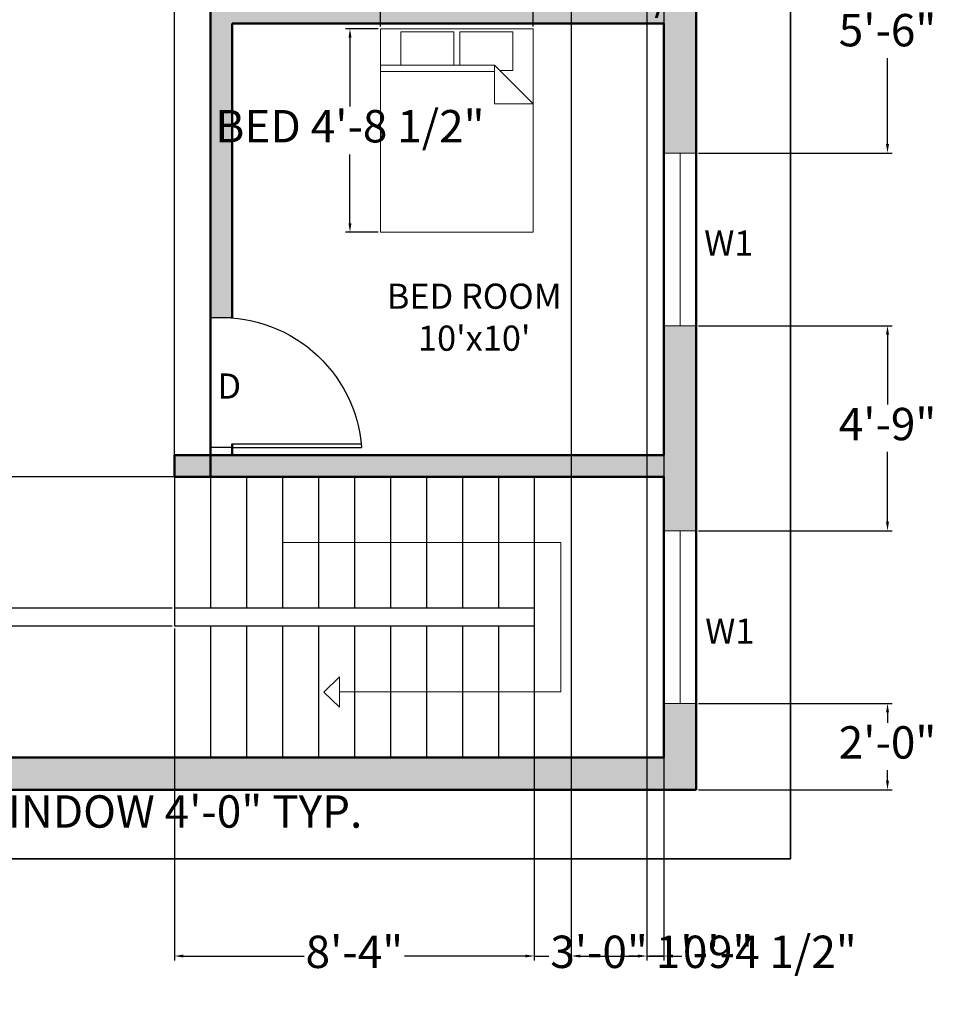
# Model space of a CAD drawing. Units: inches. Extents: x 6193 to 6719, y 6945 to 7563.
# Tile 2 of 4: x 6464 to 6719, y 6945 to 7219. Entities that reach past the tile are written whole.
import ezdxf

# ---------------------------------------------------------------- set-up
doc = ezdxf.new("R2010")
doc.units = ezdxf.units.IN
for name, color, linetype, lineweight in [('A-ANNO-DIMS', 2, 'Continuous', 18), ('A-ANNO-SYMB', 7, 'Continuous', 18), ('A-ANNO-TEXT', 7, 'Continuous', 18), ('A-ANNO-TTLB', 7, 'Continuous', 35), ('A-AREA-IDEN', 7, 'Continuous', 25), ('A-DOOR', 3, 'Continuous', 25), ('A-FLOR-STRS', 7, 'Continuous', 25), ('A-FURN', 8, 'Continuous', 18), ('A-GLAZ', 4, 'Continuous', 18), ('A-WALL', 7, 'Continuous', 50)]:
    doc.layers.add(name, color=color, linetype=linetype, lineweight=lineweight)
doc.layers.add('A-WALL-PATT', color=18, linetype='Continuous', lineweight=13, true_color=0x000000)
doc.styles.get("Standard").update_dxf_attribs({"font": 'arial.ttf'})
doc.dimstyles.new('ISO-25', dxfattribs={"dimtxt": 9, "dimasz": 2.5, "dimexe": 1.25, "dimexo": 0.625, "dimgap": 2, "dimtad": 0, "dimtih": 1, "dimtoh": 1, "dimdec": 1, "dimlunit": 4, "dimtxsty": 'Standard', "dimcen": 2.5, "dimadec": 0, "dimazin": 0, "dimtfac": 0.5, "dimtdec": 1, "dimtmove": 0, "dimatfit": 3, "dimfxl": 1, "dimarcsym": 0})

# ---------------------------------------------------------------- blocks, each defined once
blk = doc.blocks.new('Bed - Queen')
for p, q in [((0, -80.00003), (0, 0)), ((0, 0), (59.99999, 0)), ((59.99999, 0), (59.99999, -80.00003)), ((7.99999, -1.2), (28.79998, -1.2)), ((7.99999, -14.4), (7.99999, -1.2)), ((28.79998, -1.2), (28.79998, -14.4)), ((31.19999, -1.2), (51.99999, -1.2)), ((31.19999, -14.4), (31.19999, -1.2)), ((51.99999, -1.2), (51.99999, -16.4)), ((0, -14.4), (44.8, -14.4)), ((59.99999, -29.6), (44.8, -14.4)), ((44.8, -14.4), (44.8, -29.6)), ((44.8, -16.8), (0, -16.8)), ((51.99999, -16.4), (46.79936, -16.4)), ((44.8, -29.6), (59.99999, -29.6)), ((59.99999, -80.00003), (0, -80.00003))]:
    blk.add_line(p, q)
blk = doc.blocks.new('DOOR-SWING-36IN')
for p, q in [((0, 6), (0, 42)), ((1, 6), (1, 41.91)), ((0, 6), (0, 0)), ((36, 6), (36, 0))]:
    blk.add_line(p, q)
blk.add_arc((-3, 3), 39.12, 355.6013, 85.6013)
blk = doc.blocks.new('WIN-48IN')
for p, q in [((0, 48), (9, 48)), ((4.5, 48), (4.5, 0)), ((0, 0), (9, 0))]:
    blk.add_line(p, q)
blk = doc.blocks.new('*D14')
at = {"layer": 'A-ANNO-DIMS', "color": 0, "lineweight": -2, "transparency": 16777216}
for p, q in [((6395.41, 7004.04), (6395.41, 6996.21)), ((6443.41, 7004.04), (6443.41, 6996.21)), ((6397.91, 6997.46), (6440.91, 6997.46)), ((6443.41, 6997.46), (6445.91, 6997.46))]:
    blk.add_line(p, q, dxfattribs=at)
at = {"layer": 'A-ANNO-DIMS', "color": 0, "transparency": 16777216}
for points in [[(6397.91, 6997.88), (6397.91, 6997.05), (6395.41, 6997.46)], [(6440.91, 6997.88), (6440.91, 6997.05), (6443.41, 6997.46)]]:
    blk.add_solid(points, dxfattribs=at)
at = {"layer": 'Defpoints', "color": 0, "transparency": 16777216}
for p in [(6395.41, 7004.66), (6443.41, 7004.66), (6443.41, 6997.46)]:
    blk.add_point(p, dxfattribs=at)
at = {"layer": 'A-ANNO-DIMS', "color": 0, "transparency": 16777216, "insert": (6504.85, 6997.46), "char_height": 9, "attachment_point": 5}
blk.add_mtext('WINDOW 4\'-0" TYP.', dxfattribs=at)
blk = doc.blocks.new('*D18')
at = {"layer": 'A-ANNO-DIMS', "color": 0, "lineweight": -2, "transparency": 16777216}
for p, q in [((6563.91, 7216.24), (6554.8, 7216.24)), ((6556.05, 7213.74), (6556.05, 7194.61)), ((6556.05, 7162.17), (6556.05, 7181.3)), ((6563.91, 7159.67), (6554.8, 7159.67))]:
    blk.add_line(p, q, dxfattribs=at)
at = {"layer": 'A-ANNO-DIMS', "color": 0, "transparency": 16777216}
for points in [[(6555.64, 7213.74), (6556.47, 7213.74), (6556.05, 7216.24)], [(6555.64, 7162.17), (6556.47, 7162.17), (6556.05, 7159.67)]]:
    blk.add_solid(points, dxfattribs=at)
at = {"layer": 'Defpoints', "color": 0, "transparency": 16777216}
for p in [(6556.05, 7216.24), (6564.54, 7216.24), (6564.54, 7159.67)]:
    blk.add_point(p, dxfattribs=at)
at = {"layer": 'A-ANNO-DIMS', "color": 0, "transparency": 16777216, "insert": (6556.05, 7187.96), "char_height": 9, "attachment_point": 5}
blk.add_mtext('BED 4\'-8 1/2"', dxfattribs=at)
blk = doc.blocks.new('*D19')
at = {"layer": 'A-ANNO-DIMS', "color": 0, "lineweight": -2, "transparency": 16777216}
for p, q in [((6564.54, 7216.86), (6564.54, 7225.97)), ((6606.96, 7216.86), (6606.96, 7225.97)), ((6567.04, 7224.72), (6604.46, 7224.72)), ((6606.96, 7224.72), (6609.46, 7224.72))]:
    blk.add_line(p, q, dxfattribs=at)
at = {"layer": 'A-ANNO-DIMS', "color": 0, "transparency": 16777216}
for points in [[(6567.04, 7225.14), (6567.04, 7224.31), (6564.54, 7224.72)], [(6604.46, 7225.14), (6604.46, 7224.31), (6606.96, 7224.72)]]:
    blk.add_solid(points, dxfattribs=at)
at = {"layer": 'Defpoints', "color": 0, "transparency": 16777216}
for p in [(6606.96, 7224.72), (6564.54, 7216.24), (6606.96, 7216.24)]:
    blk.add_point(p, dxfattribs=at)
at = {"layer": 'A-ANNO-DIMS', "color": 0, "transparency": 16777216, "insert": (6633.91, 7224.72), "char_height": 9, "attachment_point": 5}
blk.add_mtext('3\'-6 1/2"', dxfattribs=at)
blk = doc.blocks.new('*D37')
at = {"layer": 'A-ANNO-DIMS', "color": 0, "lineweight": -2, "transparency": 16777216}
for p, q in [((6652.91, 7028.66), (6706.68, 7028.66)), ((6705.43, 7026.16), (6705.43, 7023.26)), ((6705.43, 7007.16), (6705.43, 7010.07)), ((6652.91, 7004.66), (6706.68, 7004.66))]:
    blk.add_line(p, q, dxfattribs=at)
at = {"layer": 'A-ANNO-DIMS', "color": 0, "transparency": 16777216}
for points in [[(6705.01, 7026.16), (6705.84, 7026.16), (6705.43, 7028.66)], [(6705.01, 7007.16), (6705.84, 7007.16), (6705.43, 7004.66)]]:
    blk.add_solid(points, dxfattribs=at)
at = {"layer": 'Defpoints', "color": 0, "transparency": 16777216}
for p in [(6652.28, 7028.66), (6705.43, 7028.66), (6652.28, 7004.66)]:
    blk.add_point(p, dxfattribs=at)
at = {"layer": 'A-ANNO-DIMS', "color": 0, "transparency": 16777216, "insert": (6705.43, 7016.66), "char_height": 9, "attachment_point": 5}
blk.add_mtext('2\'-0"', dxfattribs=at)
blk = doc.blocks.new('*D38')
at = {"layer": 'A-ANNO-DIMS', "color": 0, "lineweight": -2, "transparency": 16777216}
for p, q in [((6652.91, 7133.66), (6706.68, 7133.66)), ((6705.43, 7131.16), (6705.43, 7111.76)), ((6705.43, 7079.16), (6705.43, 7098.57)), ((6652.91, 7076.66), (6706.68, 7076.66))]:
    blk.add_line(p, q, dxfattribs=at)
at = {"layer": 'A-ANNO-DIMS', "color": 0, "transparency": 16777216}
for points in [[(6705.01, 7131.16), (6705.84, 7131.16), (6705.43, 7133.66)], [(6705.01, 7079.16), (6705.84, 7079.16), (6705.43, 7076.66)]]:
    blk.add_solid(points, dxfattribs=at)
at = {"layer": 'Defpoints', "color": 0, "transparency": 16777216}
for p in [(6652.28, 7133.66), (6705.43, 7133.66), (6652.28, 7076.66)]:
    blk.add_point(p, dxfattribs=at)
at = {"layer": 'A-ANNO-DIMS', "color": 0, "transparency": 16777216, "insert": (6705.43, 7105.16), "char_height": 9, "attachment_point": 5}
blk.add_mtext('4\'-9"', dxfattribs=at)
blk = doc.blocks.new('*D39')
at = {"layer": 'A-ANNO-DIMS', "color": 0, "lineweight": -2, "transparency": 16777216}
for p, q in [((6652.91, 7247.66), (6706.68, 7247.66)), ((6705.43, 7245.16), (6705.43, 7221.26)), ((6705.43, 7184.16), (6705.43, 7208.07)), ((6652.91, 7181.66), (6706.68, 7181.66))]:
    blk.add_line(p, q, dxfattribs=at)
at = {"layer": 'A-ANNO-DIMS', "color": 0, "transparency": 16777216}
for points in [[(6705.01, 7245.16), (6705.84, 7245.16), (6705.43, 7247.66)], [(6705.01, 7184.16), (6705.84, 7184.16), (6705.43, 7181.66)]]:
    blk.add_solid(points, dxfattribs=at)
at = {"layer": 'Defpoints', "color": 0, "transparency": 16777216}
for p in [(6652.28, 7247.66), (6705.43, 7247.66), (6652.28, 7181.66)]:
    blk.add_point(p, dxfattribs=at)
at = {"layer": 'A-ANNO-DIMS', "color": 0, "transparency": 16777216, "insert": (6705.43, 7214.66), "char_height": 9, "attachment_point": 5}
blk.add_mtext('5\'-6"', dxfattribs=at)
blk = doc.blocks.new('*D47')
at = {"layer": 'A-ANNO-DIMS', "color": 0, "lineweight": -2, "transparency": 16777216}
for p, q in [((6507.28, 7049.54), (6507.28, 6957.2)), ((6607.28, 7049.54), (6607.28, 6957.2)), ((6509.78, 6958.45), (6543.32, 6958.45)), ((6604.78, 6958.45), (6571.25, 6958.45))]:
    blk.add_line(p, q, dxfattribs=at)
at = {"layer": 'A-ANNO-DIMS', "color": 0, "transparency": 16777216}
for points in [[(6509.78, 6958.86), (6509.78, 6958.03), (6507.28, 6958.45)], [(6604.78, 6958.86), (6604.78, 6958.03), (6607.28, 6958.45)]]:
    blk.add_solid(points, dxfattribs=at)
at = {"layer": 'Defpoints', "color": 0, "transparency": 16777216}
for p in [(6507.28, 7050.16), (6607.28, 7050.16), (6607.28, 6958.45)]:
    blk.add_point(p, dxfattribs=at)
at = {"layer": 'A-ANNO-DIMS', "color": 0, "transparency": 16777216, "insert": (6557.28, 6958.45), "char_height": 9, "attachment_point": 5}
blk.add_mtext('8\'-4"', dxfattribs=at)
blk = doc.blocks.new('*D48')
at = {"layer": 'A-ANNO-DIMS', "color": 0, "lineweight": -2, "transparency": 16777216}
for p, q in [((6607.28, 7013.04), (6607.28, 6957.2)), ((6643.28, 7013.04), (6643.28, 6957.2)), ((6604.78, 6958.45), (6602.28, 6958.45)), ((6607.28, 6958.45), (6611.33, 6958.45)), ((6643.28, 6958.45), (6639.24, 6958.45)), ((6645.78, 6958.45), (6648.28, 6958.45))]:
    blk.add_line(p, q, dxfattribs=at)
at = {"layer": 'A-ANNO-DIMS', "color": 0, "transparency": 16777216}
for points in [[(6604.78, 6958.86), (6604.78, 6958.03), (6607.28, 6958.45)], [(6645.78, 6958.86), (6645.78, 6958.03), (6643.28, 6958.45)]]:
    blk.add_solid(points, dxfattribs=at)
at = {"layer": 'Defpoints', "color": 0, "transparency": 16777216}
for p in [(6607.28, 7013.66), (6643.28, 7013.66), (6643.28, 6958.45)]:
    blk.add_point(p, dxfattribs=at)
at = {"layer": 'A-ANNO-DIMS', "color": 0, "transparency": 16777216, "insert": (6625.28, 6958.45), "char_height": 9, "attachment_point": 5}
blk.add_mtext('3\'-0"', dxfattribs=at)
blk = doc.blocks.new('*D49')
at = {"layer": 'A-ANNO-DIMS', "color": 0, "lineweight": -2, "transparency": 16777216}
for p, q in [((6506.66, 7091.66), (6215.49, 7091.66)), ((6216.74, 7089.16), (6216.74, 7080.07)), ((6216.74, 7057.66), (6216.74, 7066.76)), ((6506.66, 7055.16), (6215.49, 7055.16))]:
    blk.add_line(p, q, dxfattribs=at)
at = {"layer": 'A-ANNO-DIMS', "color": 0, "transparency": 16777216}
for points in [[(6216.32, 7089.16), (6217.16, 7089.16), (6216.74, 7091.66)], [(6216.32, 7057.66), (6217.16, 7057.66), (6216.74, 7055.16)]]:
    blk.add_solid(points, dxfattribs=at)
at = {"layer": 'Defpoints', "color": 0, "transparency": 16777216}
for p in [(6216.74, 7091.66), (6507.28, 7091.66), (6507.28, 7055.16)]:
    blk.add_point(p, dxfattribs=at)
at = {"layer": 'A-ANNO-DIMS', "color": 0, "transparency": 16777216, "insert": (6216.74, 7073.41), "char_height": 9, "attachment_point": 5}
blk.add_mtext('3\'-0 1/2"', dxfattribs=at)
blk = doc.blocks.new('*D50')
at = {"layer": 'A-ANNO-DIMS', "color": 0, "lineweight": -2, "transparency": 16777216}
for p, q in [((6642.66, 7091.66), (6215.49, 7091.66)), ((6216.74, 7089.16), (6216.74, 7059.26)), ((6216.74, 7016.16), (6216.74, 7046.07)), ((6642.66, 7013.66), (6215.49, 7013.66))]:
    blk.add_line(p, q, dxfattribs=at)
at = {"layer": 'A-ANNO-DIMS', "color": 0, "transparency": 16777216}
for points in [[(6216.32, 7089.16), (6217.16, 7089.16), (6216.74, 7091.66)], [(6216.32, 7016.16), (6217.16, 7016.16), (6216.74, 7013.66)]]:
    blk.add_solid(points, dxfattribs=at)
at = {"layer": 'Defpoints', "color": 0, "transparency": 16777216}
for p in [(6216.74, 7091.66), (6643.28, 7091.66), (6643.28, 7013.66)]:
    blk.add_point(p, dxfattribs=at)
at = {"layer": 'A-ANNO-DIMS', "color": 0, "transparency": 16777216, "insert": (6216.74, 7052.66), "char_height": 9, "attachment_point": 5}
blk.add_mtext('6\'-6"', dxfattribs=at)
blk = doc.blocks.new('*D51')
at = {"layer": 'A-ANNO-DIMS', "color": 0, "lineweight": -2, "transparency": 16777216}
for p, q in [((6507.28, 7092.29), (6507.28, 7551.02)), ((6509.78, 7549.77), (6514.78, 7549.77)), ((6517.28, 7092.29), (6517.28, 7551.02)), ((6517.28, 7549.77), (6519.78, 7549.77))]:
    blk.add_line(p, q, dxfattribs=at)
at = {"layer": 'A-ANNO-DIMS', "color": 0, "transparency": 16777216}
for points in [[(6509.78, 7550.19), (6509.78, 7549.36), (6507.28, 7549.77)], [(6514.78, 7550.19), (6514.78, 7549.36), (6517.28, 7549.77)]]:
    blk.add_solid(points, dxfattribs=at)
at = {"layer": 'Defpoints', "color": 0, "transparency": 16777216}
for p in [(6517.28, 7549.77), (6507.28, 7091.66), (6517.28, 7091.66)]:
    blk.add_point(p, dxfattribs=at)
at = {"layer": 'A-ANNO-DIMS', "color": 0, "transparency": 16777216, "insert": (6537.24, 7549.77), "char_height": 9, "attachment_point": 5}
blk.add_mtext('0\'-10"', dxfattribs=at)
blk = doc.blocks.new('*D52')
at = {"layer": 'A-ANNO-DIMS', "color": 0, "lineweight": -2, "transparency": 16777216}
for p, q in [((6216.74, 7057.66), (6216.74, 7060.16)), ((6216.74, 7060.16), (6219.24, 7060.16)), ((6506.66, 7055.16), (6215.49, 7055.16)), ((6216.74, 7050.16), (6216.74, 7055.16)), ((6506.66, 7050.16), (6215.49, 7050.16)), ((6216.74, 7047.66), (6216.74, 7045.16))]:
    blk.add_line(p, q, dxfattribs=at)
at = {"layer": 'A-ANNO-DIMS', "color": 0, "transparency": 16777216}
for points in [[(6216.32, 7057.66), (6217.16, 7057.66), (6216.74, 7055.16)], [(6216.32, 7047.66), (6217.16, 7047.66), (6216.74, 7050.16)]]:
    blk.add_solid(points, dxfattribs=at)
at = {"layer": 'Defpoints', "color": 0, "transparency": 16777216}
for p in [(6216.74, 7055.16), (6507.28, 7055.16), (6507.28, 7050.16)]:
    blk.add_point(p, dxfattribs=at)
at = {"layer": 'A-ANNO-DIMS', "color": 0, "transparency": 16777216, "insert": (6233.2, 7060.16), "char_height": 9, "attachment_point": 5}
blk.add_mtext('0\'-5"', dxfattribs=at)
blk = doc.blocks.new('*D54')
at = {"layer": 'A-ANNO-DIMS', "color": 0, "lineweight": -2, "transparency": 16777216}
for p, q in [((6617.56, 7223.04), (6617.56, 6957.2)), ((6638.56, 7223.04), (6638.56, 6957.2)), ((6620.06, 6958.45), (6636.06, 6958.45)), ((6638.56, 6958.45), (6641.06, 6958.45))]:
    blk.add_line(p, q, dxfattribs=at)
at = {"layer": 'A-ANNO-DIMS', "color": 0, "transparency": 16777216}
for points in [[(6620.06, 6958.86), (6620.06, 6958.03), (6617.56, 6958.45)], [(6636.06, 6958.86), (6636.06, 6958.03), (6638.56, 6958.45)]]:
    blk.add_solid(points, dxfattribs=at)
at = {"layer": 'Defpoints', "color": 0, "transparency": 16777216}
for p in [(6617.56, 7223.66), (6638.56, 7223.66), (6638.56, 6958.45)]:
    blk.add_point(p, dxfattribs=at)
at = {"layer": 'A-ANNO-DIMS', "color": 0, "transparency": 16777216, "insert": (6654.6, 6958.45), "char_height": 9, "attachment_point": 5}
blk.add_mtext('1\'-9"', dxfattribs=at)
blk = doc.blocks.new('*D56')
at = {"layer": 'A-ANNO-DIMS', "color": 0, "lineweight": -2, "transparency": 16777216}
for p, q in [((6638.56, 7223.04), (6638.56, 6957.2)), ((6643.28, 7223.04), (6643.28, 6957.2)), ((6636.06, 6958.45), (6633.56, 6958.45)), ((6638.56, 6958.45), (6643.28, 6958.45)), ((6645.78, 6958.45), (6648.28, 6958.45))]:
    blk.add_line(p, q, dxfattribs=at)
at = {"layer": 'A-ANNO-DIMS', "color": 0, "transparency": 16777216}
for points in [[(6636.06, 6958.86), (6636.06, 6958.03), (6638.56, 6958.45)], [(6645.78, 6958.86), (6645.78, 6958.03), (6643.28, 6958.45)]]:
    blk.add_solid(points, dxfattribs=at)
at = {"layer": 'Defpoints', "color": 0, "transparency": 16777216}
for p in [(6638.56, 7223.66), (6643.28, 7223.66), (6643.28, 6958.45)]:
    blk.add_point(p, dxfattribs=at)
at = {"layer": 'A-ANNO-DIMS', "color": 0, "transparency": 16777216, "insert": (6672.73, 6958.45), "char_height": 9, "attachment_point": 5}
blk.add_mtext('0\'-4 1/2"', dxfattribs=at)

msp = doc.modelspace()

# ---------------------------------------------------------------- hatches: boundary and pattern name
at = {"layer": 'A-WALL-PATT'}
h = msp.add_hatch(color=256, dxfattribs=at)
h.dxf.hatch_style = 1
h.paths.add_polyline_path([(6529.28, 7484.66), (6292.28, 7484.66), (6292.28, 7436.66), (6301.28, 7436.66), (6301.28, 7475.66), (6469.28, 7475.66), (6469.28, 7295.66), (6475.28, 7295.66), (6479.73, 7295.66), (6479.73, 7301.66), (6475.28, 7301.66), (6475.28, 7475.66), (6529.28, 7475.66)])
h.paths.add_polyline_path([(6652.28, 7484.66), (6589.28, 7484.66), (6589.28, 7475.66), (6643.28, 7475.66), (6643.28, 7412.66), (6652.28, 7412.66)])
h.paths.add_polyline_path([(6652.28, 7364.66), (6643.28, 7364.66), (6643.28, 7301.66), (6515.73, 7301.66, -0.038405), (6515.73, 7295.66), (6565.28, 7295.66), (6565.28, 7248.66, -0.055385), (6571.28, 7248.66), (6571.28, 7295.66), (6643.28, 7295.66), (6643.28, 7271.66), (6652.28, 7271.66)])
h.paths.add_polyline_path([(6652.28, 7247.66), (6643.28, 7247.66), (6643.28, 7223.66), (6571.28, 7223.66), (6565.28, 7223.66), (6517.28, 7223.66), (6517.28, 7217.66), (6517.28, 7135.82, -0.038405), (6523.28, 7135.82), (6523.28, 7217.66), (6565.28, 7217.66), (6571.28, 7217.66), (6643.28, 7217.66), (6643.28, 7181.66), (6652.28, 7181.66)])
h.paths.add_polyline_path([(6301.28, 7217.66), (6410.54, 7217.66), (6410.54, 7223.66), (6301.28, 7223.66), (6301.28, 7259.66), (6292.28, 7259.66), (6292.28, 7139.66), (6301.28, 7139.66)])
h.paths.add_polyline_path([(6301.28, 7343.66), (6361.63, 7343.66), (6361.63, 7349.66), (6301.28, 7349.66), (6301.28, 7388.66), (6292.28, 7388.66), (6292.28, 7307.66), (6301.28, 7307.66)], flags=17)
h.paths.add_polyline_path([(6301.28, 7091.66), (6292.28, 7091.66), (6292.28, 7004.66), (6302.28, 7004.66), (6302.28, 7013.66), (6301.28, 7013.66)])
h.paths.add_polyline_path([(6395.41, 7013.66), (6338.28, 7013.66, -0.055385), (6338.28, 7004.66), (6395.41, 7004.66)])
h.paths.add_polyline_path([(6652.28, 7028.66), (6643.28, 7028.66), (6643.28, 7013.66), (6443.41, 7013.66), (6443.41, 7004.66), (6652.28, 7004.66)])
h.paths.add_polyline_path([(6652.28, 7133.66), (6643.28, 7133.66), (6643.28, 7097.66), (6523.28, 7097.66), (6517.28, 7097.66), (6517.28, 7091.66), (6523.28, 7091.66), (6643.28, 7091.66), (6643.28, 7076.66), (6652.28, 7076.66)])
h.paths.add_polyline_path([(6517.28, 7097.66), (6507.28, 7097.66), (6507.28, 7091.66), (6517.28, 7091.66)])

# ---------------------------------------------------------------- linework, layer by layer
at = {"layer": 'A-ANNO-SYMB'}
for p, q in [((6537.28, 7073.41), (6614.67, 7073.41)), ((6614.67, 7073.41), (6614.67, 7031.91)), ((6548.78, 7031.84), (6553.17, 7036.08)), ((6553.17, 7031.91), (6553.17, 7036.08)), ((6553.17, 7036.08), (6553.17, 7027.59)), ((6553.17, 7027.59), (6548.78, 7031.84)), ((6557.28, 7031.91), (6553.17, 7031.91)), ((6557.28, 7031.91), (6614.67, 7031.91))]:
    msp.add_line(p, q, dxfattribs=at)
at = {"layer": 'A-ANNO-TTLB'}
msp.add_lwpolyline([(6243.74, 7522.77), (6678.43, 7522.77), (6678.43, 6985.45), (6243.74, 6985.45)], close=True, dxfattribs=at)
at = {"layer": 'A-FLOR-STRS'}
for p, q in [((6507.28, 7091.66), (6507.28, 7050.16)), ((6517.28, 7091.66), (6517.28, 7055.16)), ((6527.28, 7091.66), (6527.28, 7055.16)), ((6537.28, 7091.66), (6537.28, 7055.16)), ((6547.28, 7091.66), (6547.28, 7055.16)), ((6557.28, 7091.66), (6557.28, 7055.16)), ((6567.28, 7091.66), (6567.28, 7055.16)), ((6577.28, 7091.66), (6577.28, 7055.16)), ((6587.28, 7091.66), (6587.28, 7055.16)), ((6597.28, 7091.66), (6597.28, 7055.16)), ((6607.28, 7091.66), (6607.28, 7013.66)), ((6517.28, 7055.16), (6507.28, 7055.16)), ((6607.28, 7055.16), (6517.28, 7055.16)), ((6517.28, 7050.16), (6507.28, 7050.16)), ((6607.28, 7050.16), (6517.28, 7050.16)), ((6517.28, 7050.16), (6517.28, 7013.66)), ((6527.28, 7050.16), (6527.28, 7013.66)), ((6537.28, 7050.16), (6537.28, 7013.66)), ((6547.28, 7050.16), (6547.28, 7013.66)), ((6557.28, 7050.16), (6557.28, 7013.66)), ((6567.28, 7050.16), (6567.28, 7013.66)), ((6577.28, 7050.16), (6577.28, 7013.66)), ((6587.28, 7050.16), (6587.28, 7013.66)), ((6597.28, 7050.16), (6597.28, 7013.66))]:
    msp.add_line(p, q, dxfattribs=at)
at = {"layer": 'A-WALL'}
for p, q in [((6652.28, 7484.66), (6652.28, 7004.66)), ((6517.28, 7217.66), (6517.28, 7223.66)), ((6517.28, 7217.66), (6517.28, 7097.66)), ((6523.28, 7217.66), (6523.28, 7135.82)), ((6565.28, 7217.66), (6523.28, 7217.66)), ((6571.28, 7217.66), (6565.28, 7217.66)), ((6571.28, 7217.66), (6643.28, 7217.66)), ((6643.28, 7217.66), (6643.28, 7097.66)), ((6523.28, 7100.82), (6523.28, 7097.66)), ((6517.28, 7097.66), (6507.28, 7097.66)), ((6507.28, 7091.66), (6507.28, 7097.66)), ((6517.28, 7097.66), (6517.28, 7091.66)), ((6523.28, 7097.66), (6517.28, 7097.66)), ((6523.28, 7097.66), (6643.28, 7097.66)), ((6517.28, 7091.66), (6507.28, 7091.66)), ((6523.28, 7091.66), (6517.28, 7091.66)), ((6523.28, 7091.66), (6643.28, 7091.66)), ((6643.28, 7091.66), (6643.28, 7013.66)), ((6643.28, 7013.66), (6338.28, 7013.66)), ((6652.28, 7004.66), (6338.28, 7004.66))]:
    msp.add_line(p, q, dxfattribs=at)

# ---------------------------------------------------------------- block references
at = {"layer": 'A-DOOR', "extrusion": (0, 0, -1), "zscale": -1, "rotation": 90.0000000000012}
msp.add_blockref('DOOR-SWING-36IN', (-6517.28, 7099.82), dxfattribs=at)
at = {"layer": 'A-FURN', "xscale": 0.7070706530272395, "yscale": 0.7070706530272395, "zscale": 0.7070706530272395}
msp.add_blockref('Bed - Queen', (6564.54, 7216.24), dxfattribs=at)
at = {"layer": 'A-GLAZ'}
for p in [(6643.28, 7133.66), (6643.28, 7028.66)]:
    msp.add_blockref('WIN-48IN', p, dxfattribs=at)

# ---------------------------------------------------------------- texts
at = {"layer": 'A-ANNO-TEXT', "char_height": 7, "attachment_point": 1}
for s, width, insert in [('\\pxqc;W1', 21.3946, (6650.62, 7160.15)), ('\\pxqc;D', 20.1481, (6512.43, 7120.39)), ('\\pxqc;W1', 21.3946, (6650.9, 7052.27))]:
    msp.add_mtext_dynamic_manual_height_columns(s, width=width, gutter_width=12.5, heights=[0], dxfattribs=dict(at, insert=insert))
at = {"layer": 'A-AREA-IDEN', "insert": (6555.94, 7145.37), "char_height": 7, "attachment_point": 1}
msp.add_mtext_dynamic_manual_height_columns("\\pxqc;{\\fArial|b1|i0|c0|p34;BED ROOM\\P10'x10'}", width=69.2902, gutter_width=12.5, heights=[0], dxfattribs=at)

# ---------------------------------------------------------------- dimensions: what is measured, and where the dimension line sits
at = {"layer": 'A-ANNO-DIMS'}
for base, p1, p2, picture, middle in [((6517.28, 7549.77), (6507.28, 7091.66), (6517.28, 7091.66), '*D51', (6537.24, 7549.77)), ((6606.96, 7224.72), (6564.54, 7216.24), (6606.96, 7216.24), '*D19', (6633.91, 7224.72)), ((6638.56, 6958.45), (6617.56, 7223.66), (6638.56, 7223.66), '*D54', (6654.6, 6958.45)), ((6643.28, 6958.45), (6638.56, 7223.66), (6643.28, 7223.66), '*D56', (6672.73, 6958.45)), ((6607.28, 6958.45), (6507.28, 7050.16), (6607.28, 7050.16), '*D47', (6557.28, 6958.45)), ((6643.28, 6958.45), (6607.28, 7013.66), (6643.28, 7013.66), '*D48', (6625.28, 6958.45))]:
    dim = msp.add_linear_dim(base=base, p1=p1, p2=p2, dimstyle='ISO-25', override={"dimdec": 1, "dimlfac": 1, "dimrnd": 0, "dimzin": 1, "dimdsep": 46, "dimlunit": 4, "dimfrac": 2}, dxfattribs=at)
    dim.commit()
    dim.dimension.update_dxf_attribs({"geometry": picture, "text_midpoint": middle})
for base, p1, p2, picture, middle in [((6705.43, 7247.66), (6652.28, 7181.66), (6652.28, 7247.66), '*D39', (6705.43, 7214.66)), ((6705.43, 7133.66), (6652.28, 7076.66), (6652.28, 7133.66), '*D38', (6705.43, 7105.16)), ((6216.74, 7091.66), (6507.28, 7055.16), (6507.28, 7091.66), '*D49', (6216.74, 7073.41)), ((6216.74, 7091.66), (6643.28, 7013.66), (6643.28, 7091.66), '*D50', (6216.74, 7052.66)), ((6216.74, 7055.16), (6507.28, 7050.16), (6507.28, 7055.16), '*D52', (6233.2, 7060.16)), ((6705.43, 7028.66), (6652.28, 7004.66), (6652.28, 7028.66), '*D37', (6705.43, 7016.66))]:
    dim = msp.add_linear_dim(base=base, p1=p1, p2=p2, angle=90, dimstyle='ISO-25', override={"dimdec": 1, "dimlfac": 1, "dimrnd": 0, "dimzin": 1, "dimdsep": 46, "dimlunit": 4, "dimfrac": 2}, dxfattribs=at)
    dim.commit()
    dim.dimension.update_dxf_attribs({"geometry": picture, "text_midpoint": middle})
dim = msp.add_linear_dim(base=(6556.05, 7216.24), p1=(6564.54, 7159.67), p2=(6564.54, 7216.24), angle=90, text='BED <>', dimstyle='ISO-25', override={"dimdec": 1, "dimlfac": 1, "dimrnd": 0, "dimzin": 1, "dimdsep": 46, "dimlunit": 4, "dimfrac": 2}, dxfattribs=at)
dim.commit()
dim.dimension.update_dxf_attribs({"geometry": '*D18', "text_midpoint": (6556.05, 7187.96)})
dim = msp.add_linear_dim(base=(6443.41, 6997.46), p1=(6395.41, 7004.66), p2=(6443.41, 7004.66), text='WINDOW <> TYP.', dimstyle='ISO-25', override={"dimdec": 1, "dimlfac": 1, "dimrnd": 0, "dimzin": 1, "dimdsep": 46, "dimlunit": 4, "dimfrac": 2}, dxfattribs=at)
dim.commit()
dim.dimension.update_dxf_attribs({"geometry": '*D14', "text_midpoint": (6504.85, 6997.46)})

doc.saveas('drawing.dxf')
